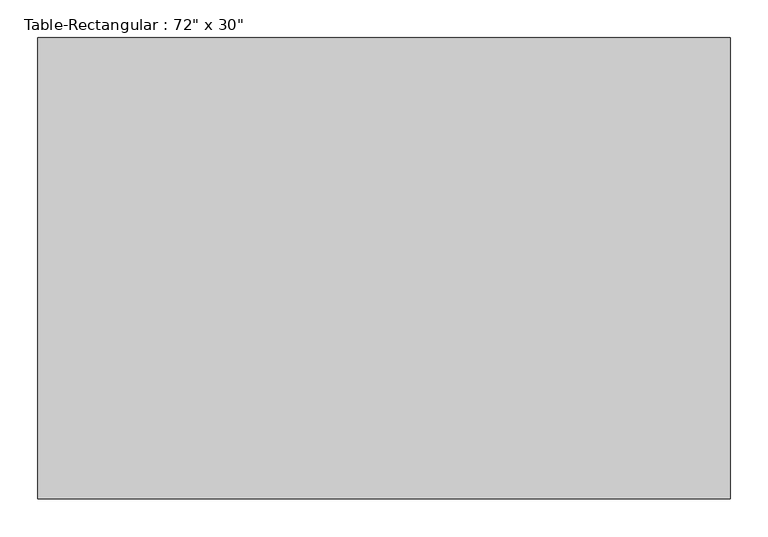
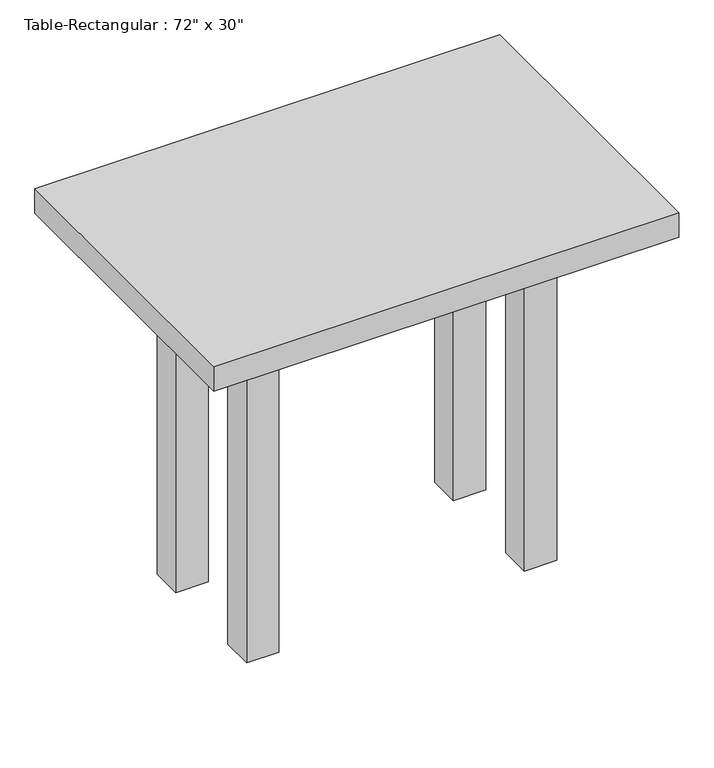
"""IFC4 building model written with IfcOpenShell, lengths in millimetres: furniture geometry."""

from ifc_helpers import new_model, si_unit, frame, origin, origin_with_axes, place, context, project, spatial, polyline, outline, extrude, source, transform, mapped, element, save


def furniture_a672282c(model_context):
    return source(origin(), model_context, "Body", "SweptSolid", [
        extrude(outline(polyline([(241.3, 114.3), (241.3, 88.9), (-241.3, 88.9), (-241.3, 114.3), (241.3, 114.3)])), frame((0.0, 0.0, 609.6), z_axis=(0.0, 0.0, 1.0), x_axis=(1.0, 0.0, 0.0)), (0.0, 0.0, 1.0), 101.6),
        extrude(outline(polyline([(241.3, -114.3), (-241.3, -114.3), (-241.3, -88.9), (241.3, -88.9), (241.3, -114.3)])), frame((0.0, 0.0, 609.6), z_axis=(0.0, 0.0, 1.0), x_axis=(1.0, 0.0, 0.0)), (0.0, 0.0, 1.0), 101.6),
        extrude(outline(polyline([(-254.0, -88.9), (-279.4, -88.9), (-279.4, 88.9), (-254.0, 88.9), (-254.0, -88.9)])), frame((0.0, 0.0, 609.6), z_axis=(0.0, 0.0, 1.0), x_axis=(1.0, 0.0, 0.0)), (0.0, 0.0, 1.0), 101.6),
        extrude(outline(polyline([(254.0, -88.9), (254.0, 88.9), (279.4, 88.9), (279.4, -88.9), (254.0, -88.9)])), frame((0.0, 0.0, 609.6), z_axis=(0.0, 0.0, 1.0), x_axis=(1.0, 0.0, 0.0)), (0.0, 0.0, 1.0), 101.6),
        extrude(outline(polyline([(457.2, 304.8), (457.2, -304.8), (-457.2, -304.8), (-457.2, 304.8), (457.2, 304.8)])), frame((0.0, 0.0, 711.2), z_axis=(0.0, 0.0, 1.0), x_axis=(1.0, 0.0, 0.0)), (0.0, 0.0, 1.0), 50.8),
        extrude(outline(polyline([(-241.3, 152.4), (-241.3, 88.9), (-304.8, 88.9), (-304.8, 152.4), (-241.3, 152.4)])), origin_with_axes(), (0.0, 0.0, 1.0), 711.2),
        extrude(outline(polyline([(241.3, 152.4), (304.8, 152.4), (304.8, 88.9), (241.3, 88.9), (241.3, 152.4)])), origin_with_axes(), (0.0, 0.0, 1.0), 711.2),
        extrude(outline(polyline([(-241.3, -152.4), (-304.8, -152.4), (-304.8, -88.9), (-241.3, -88.9), (-241.3, -152.4)])), origin_with_axes(), (0.0, 0.0, 1.0), 711.2),
        extrude(outline(polyline([(241.3, -152.4), (241.3, -88.9), (304.8, -88.9), (304.8, -152.4), (241.3, -152.4)])), origin_with_axes(), (0.0, 0.0, 1.0), 711.2),
    ])


if __name__ == "__main__":
    model = new_model("IFC4")
    model_context = context("Model", 3, world=origin())
    ifc_project = project(units=[si_unit("LENGTHUNIT", "METRE", prefix="MILLI")], contexts=[model_context])
    site = spatial("IfcSite", under=ifc_project)
    building = spatial("IfcBuilding", under=site)
    placement = place(None, origin())
    furniture_shape = furniture_a672282c(model_context)
    element("IfcFurniture", 1, ObjectType="Table-Rectangular : 72\" x 30\"", at=placement, inside=building, context=model_context, shape_type="MappedRepresentation", body=[
        mapped(furniture_shape, transform((0.0, 0.0, 0.0), x_axis=(1.0, 0.0, 0.0), y_axis=(0.0, 1.0, 0.0), z_axis=(0.0, 0.0, 1.0))),
    ])
    save(model, "model.ifc")

# Revit data of these elements
# Type "Table-Rectangular : 72\" x 30\""
#   Assembly Code = "E2020200"
#   Height = 2' - 6"
#   Length = 3' - 0"
#   Width = 2' - 0"
#   Base Material = Birch
#   Top Material = Birch
#   Default Elevation = 0
# Element 1 (IfcFurniture, "Table-Rectangular : 72\" x 30\"")
#   Materials on its faces: "Birch"
# Materials
#   "Birch": class "Wood", colour RGB 224 178 126, transparency 0, Description = "Betula Alleghaniensis", Cost = 0
